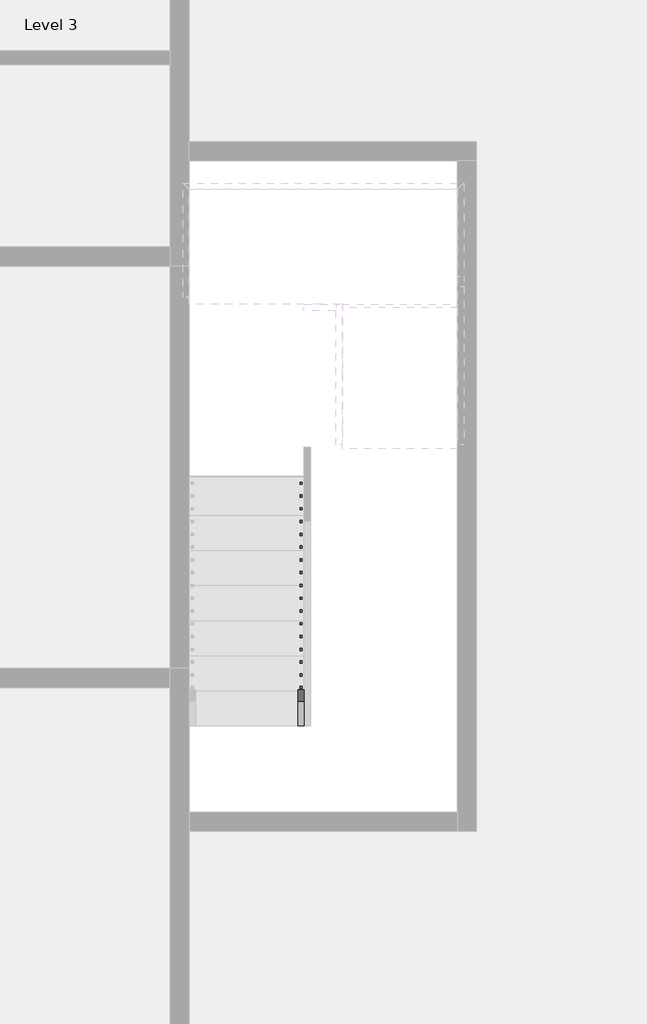
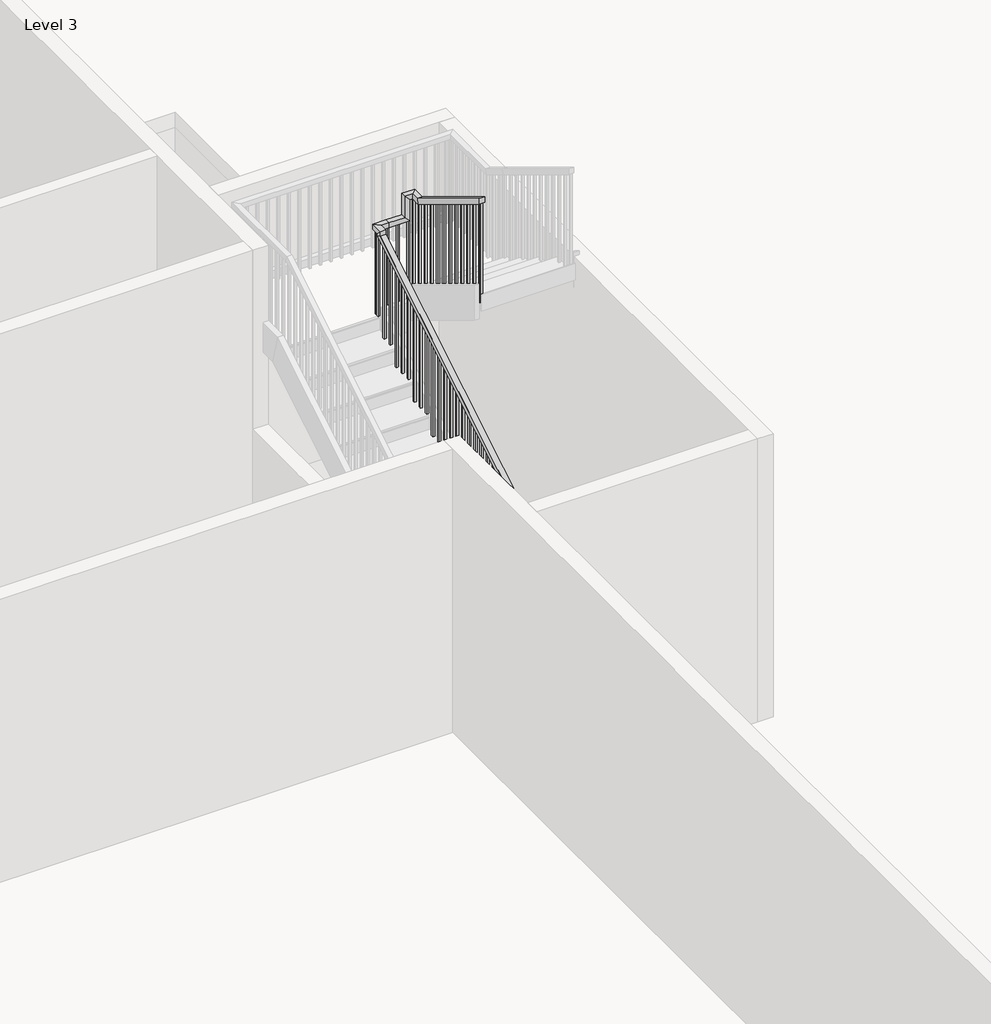
# One storey, part 7 of 8: 1 railing.
"""IFC4 building model written with IfcOpenShell, lengths in millimetres."""

from ifc_helpers import new_model, si_unit, frame, origin, place, context, project, spatial, polyline, outline, extrude, faceted_brep, element, save

model = new_model("IFC4")

# Units and contexts
model_context = context("Model", 3, world=origin())
ifc_project = project(units=[si_unit("LENGTHUNIT", "METRE", prefix="MILLI")], contexts=[model_context])

# Site, building, storey
site = spatial("IfcSite", under=ifc_project)
building = spatial("IfcBuilding", under=site)
storey = spatial("IfcBuildingStorey", under=building, Name="Level 3", Elevation=31330.6172466)

# Railing
placement = place(None, origin())
element("IfcRailing", 1, ObjectType="Handrail - Rectangular", at=placement, inside=storey, context=model_context, shape_type="SolidModel", body=[
    faceted_brep([(-2753.8415084, 19841.9216096, 32414.3505799), (-2753.8415084, 19841.9216096, 32354.9491197), (-2703.0415084, 19841.9216096, 32354.9491197), (-2703.0415084, 19841.9216096, 32414.3505799), (-2753.8415084, 23118.5216096, 34400.1687618), (-2753.8415084, 23169.3216096, 34371.5551803), (-2703.0415084, 23169.3216096, 34371.5551803), (-2703.0415084, 23118.5216096, 34400.1687618), (-2753.8415084, 23118.5216096, 34446.3505799), (-2753.8415084, 23169.3216096, 34395.5505799), (-2703.0415084, 23169.3216096, 34395.5505799), (-2703.0415084, 23118.5216096, 34446.3505799), (-2753.8415084, 23245.5216096, 34446.3505799), (-2753.8415084, 23245.5216096, 34395.5505799), (-2703.0415084, 23194.7216096, 34395.5505799), (-2703.0415084, 23194.7216096, 34446.3505799), (-2626.8415084, 23245.5216096, 34446.3505799), (-2626.8415084, 23245.5216096, 34395.5505799), (-2626.8415084, 23194.7216096, 34395.5505799), (-2626.8415084, 23194.7216096, 34446.3505799), (-2474.4415084, 23245.5216096, 34446.3505799), (-2423.6415084, 23245.5216096, 34395.5505799), (-2423.6415084, 23194.7216096, 34395.5505799), (-2474.4415084, 23194.7216096, 34446.3505799), (-2474.4415084, 23245.5216096, 34661.8657314), (-2423.6415084, 23245.5216096, 34611.0657314), (-2423.6415084, 23194.7216096, 34611.0657314), (-2474.4415084, 23194.7216096, 34661.8657314), (-2347.4415084, 23245.5216096, 34661.8657314), (-2347.4415084, 23245.5216096, 34611.0657314), (-2398.2415084, 23194.7216096, 34611.0657314), (-2398.2415084, 23194.7216096, 34661.8657314), (-2347.4415084, 23118.5216096, 34661.8657314), (-2347.4415084, 23104.3292002, 34611.0657314), (-2398.2415084, 23104.3292002, 34611.0657314), (-2398.2415084, 23118.5216096, 34661.8657314), (-2347.4415084, 22077.1216096, 35293.0172466), (-2398.2415084, 22077.1216096, 35293.0172466), (-2398.2415084, 22077.1216096, 35233.6157863), (-2347.4415084, 22077.1216096, 35233.6157863)], [[[0, 1, 2, 3]], [[1, 0, 4, 5]], [[2, 1, 5, 6]], [[3, 2, 6, 7]], [[0, 3, 7, 4]], [[5, 4, 8, 9]], [[6, 5, 9, 10]], [[7, 6, 10, 11]], [[4, 7, 11, 8]], [[9, 8, 12, 13]], [[10, 9, 13, 14]], [[11, 10, 14, 15]], [[8, 11, 15, 12]], [[13, 12, 16, 17]], [[14, 13, 17, 18]], [[15, 14, 18, 19]], [[12, 15, 19, 16]], [[17, 16, 20, 21]], [[18, 17, 21, 22]], [[19, 18, 22, 23]], [[16, 19, 23, 20]], [[21, 20, 24, 25]], [[22, 21, 25, 26]], [[23, 22, 26, 27]], [[20, 23, 27, 24]], [[25, 24, 28, 29]], [[26, 25, 29, 30]], [[27, 26, 30, 31]], [[24, 27, 31, 28]], [[29, 28, 32, 33]], [[30, 29, 33, 34]], [[31, 30, 34, 35]], [[28, 31, 35, 32]], [[36, 37, 38, 39]], [[33, 32, 36, 39]], [[34, 33, 39, 38]], [[35, 34, 38, 37]], [[32, 35, 37, 36]]]),
    extrude(outline(polyline([(22092.9966096, 35223.9945742), (22112.0466096, 35212.4491197), (22112.0466096, 34209.2839133), (22092.9966096, 34209.2839133), (22092.9966096, 35223.9945742)])), frame((-2382.3665084, 0.0, 0.0), z_axis=(1.0, 0.0, 0.0), x_axis=(0.0, 1.0, 0.0)), (0.0, 0.0, 1.0), 19.05),
    extrude(outline(polyline([(22194.5966096, 35162.4188166), (22213.6466096, 35150.8733621), (22213.6466096, 34209.2839133), (22194.5966096, 34209.2839133), (22194.5966096, 35162.4188166)])), frame((-2382.3665084, 0.0, 0.0), z_axis=(1.0, 0.0, 0.0), x_axis=(0.0, 1.0, 0.0)), (0.0, 0.0, 1.0), 19.05),
    extrude(outline(polyline([(22296.1966096, 35100.8430591), (22315.2466096, 35089.2976045), (22315.2466096, 34209.2839133), (22296.1966096, 34209.2839133), (22296.1966096, 35100.8430591)])), frame((-2382.3665084, 0.0, 0.0), z_axis=(1.0, 0.0, 0.0), x_axis=(0.0, 1.0, 0.0)), (0.0, 0.0, 1.0), 19.05),
    extrude(outline(polyline([(22397.7966096, 35039.2673015), (22416.8466096, 35027.721847), (22416.8466096, 34039.9505799), (22397.7966096, 34039.9505799), (22397.7966096, 35039.2673015)])), frame((-2382.3665084, 0.0, 0.0), z_axis=(1.0, 0.0, 0.0), x_axis=(0.0, 1.0, 0.0)), (0.0, 0.0, 1.0), 19.05),
    extrude(outline(polyline([(22499.3966096, 34977.6915439), (22518.4466096, 34966.1460894), (22518.4466096, 34039.9505799), (22499.3966096, 34039.9505799), (22499.3966096, 34977.6915439)])), frame((-2382.3665084, 0.0, 0.0), z_axis=(1.0, 0.0, 0.0), x_axis=(0.0, 1.0, 0.0)), (0.0, 0.0, 1.0), 19.05),
    extrude(outline(polyline([(22600.9966096, 34916.1157863), (22620.0466096, 34904.5703318), (22620.0466096, 34039.9505799), (22600.9966096, 34039.9505799), (22600.9966096, 34916.1157863)])), frame((-2382.3665084, 0.0, 0.0), z_axis=(1.0, 0.0, 0.0), x_axis=(0.0, 1.0, 0.0)), (0.0, 0.0, 1.0), 19.05),
    extrude(outline(polyline([(22702.5966096, 34854.5400288), (22721.6466096, 34842.9945742), (22721.6466096, 33870.6172466), (22702.5966096, 33870.6172466), (22702.5966096, 34854.5400288)])), frame((-2382.3665084, 0.0, 0.0), z_axis=(1.0, 0.0, 0.0), x_axis=(0.0, 1.0, 0.0)), (0.0, 0.0, 1.0), 19.05),
    extrude(outline(polyline([(22804.1966096, 34792.9642712), (22823.2466096, 34781.4188166), (22823.2466096, 33870.6172466), (22804.1966096, 33870.6172466), (22804.1966096, 34792.9642712)])), frame((-2382.3665084, 0.0, 0.0), z_axis=(1.0, 0.0, 0.0), x_axis=(0.0, 1.0, 0.0)), (0.0, 0.0, 1.0), 19.05),
    extrude(outline(polyline([(22905.7966096, 34731.3885136), (22924.8466096, 34719.8430591), (22924.8466096, 33870.6172466), (22905.7966096, 33870.6172466), (22905.7966096, 34731.3885136)])), frame((-2382.3665084, 0.0, 0.0), z_axis=(1.0, 0.0, 0.0), x_axis=(0.0, 1.0, 0.0)), (0.0, 0.0, 1.0), 19.05),
    extrude(outline(polyline([(23007.3966096, 34669.812756), (23026.4466096, 34658.2673015), (23026.4466096, 33701.2839133), (23007.3966096, 33701.2839133), (23007.3966096, 34669.812756)])), frame((-2382.3665084, 0.0, 0.0), z_axis=(1.0, 0.0, 0.0), x_axis=(0.0, 1.0, 0.0)), (0.0, 0.0, 1.0), 19.05),
    extrude(outline(polyline([(23108.9966096, 34608.2369985), (23128.0466096, 34596.6915439), (23128.0466096, 33701.2839133), (23108.9966096, 33701.2839133), (23108.9966096, 34608.2369985)])), frame((-2382.3665084, 0.0, 0.0), z_axis=(1.0, 0.0, 0.0), x_axis=(0.0, 1.0, 0.0)), (0.0, 0.0, 1.0), 19.05),
    extrude(outline(polyline([(-2433.1665084, 23210.5966096), (-2433.1665084, 23229.6466096), (-2414.1165084, 23229.6466096), (-2414.1165084, 23210.5966096), (-2433.1665084, 23210.5966096)])), frame((0.0, 0.0, 33531.9505799), z_axis=(0.0, 0.0, 1.0), x_axis=(1.0, 0.0, 0.0)), (0.0, 0.0, 1.0), 1079.1151515),
    extrude(outline(polyline([(-2534.7665084, 23210.5966096), (-2534.7665084, 23229.6466096), (-2515.7165084, 23229.6466096), (-2515.7165084, 23210.5966096), (-2534.7665084, 23210.5966096)])), frame((0.0, 0.0, 33531.9505799), z_axis=(0.0, 0.0, 1.0), x_axis=(1.0, 0.0, 0.0)), (0.0, 0.0, 1.0), 863.6),
    extrude(outline(polyline([(-2636.3665084, 23210.5966096), (-2636.3665084, 23229.6466096), (-2617.3165084, 23229.6466096), (-2617.3165084, 23210.5966096), (-2636.3665084, 23210.5966096)])), frame((0.0, 0.0, 33531.9505799), z_axis=(0.0, 0.0, 1.0), x_axis=(1.0, 0.0, 0.0)), (0.0, 0.0, 1.0), 863.6),
    extrude(outline(polyline([(-2718.9165084, 23185.1966096), (-2737.9665084, 23185.1966096), (-2737.9665084, 23204.2466096), (-2718.9165084, 23204.2466096), (-2718.9165084, 23185.1966096)])), frame((0.0, 0.0, 33531.9505799), z_axis=(0.0, 0.0, 1.0), x_axis=(1.0, 0.0, 0.0)), (0.0, 0.0, 1.0), 863.6),
    extrude(outline(polyline([(23083.5966096, 34319.6006348), (23102.6466096, 34331.1460894), (23102.6466096, 33362.6172466), (23083.5966096, 33362.6172466), (23083.5966096, 34319.6006348)])), frame((-2737.9665084, 0.0, 0.0), z_axis=(1.0, 0.0, 0.0), x_axis=(0.0, 1.0, 0.0)), (0.0, 0.0, 1.0), 19.05),
    extrude(outline(polyline([(22981.9966096, 34258.0248773), (23001.0466096, 34269.5703318), (23001.0466096, 33362.6172466), (22981.9966096, 33362.6172466), (22981.9966096, 34258.0248773)])), frame((-2737.9665084, 0.0, 0.0), z_axis=(1.0, 0.0, 0.0), x_axis=(0.0, 1.0, 0.0)), (0.0, 0.0, 1.0), 19.05),
    extrude(outline(polyline([(22880.3966096, 34196.4491197), (22899.4466096, 34207.9945742), (22899.4466096, 33193.2839133), (22880.3966096, 33193.2839133), (22880.3966096, 34196.4491197)])), frame((-2737.9665084, 0.0, 0.0), z_axis=(1.0, 0.0, 0.0), x_axis=(0.0, 1.0, 0.0)), (0.0, 0.0, 1.0), 19.05),
    extrude(outline(polyline([(22778.7966096, 34134.8733621), (22797.8466096, 34146.4188166), (22797.8466096, 33193.2839133), (22778.7966096, 33193.2839133), (22778.7966096, 34134.8733621)])), frame((-2737.9665084, 0.0, 0.0), z_axis=(1.0, 0.0, 0.0), x_axis=(0.0, 1.0, 0.0)), (0.0, 0.0, 1.0), 19.05),
    extrude(outline(polyline([(22677.1966096, 34073.2976045), (22696.2466096, 34084.8430591), (22696.2466096, 33193.2839133), (22677.1966096, 33193.2839133), (22677.1966096, 34073.2976045)])), frame((-2737.9665084, 0.0, 0.0), z_axis=(1.0, 0.0, 0.0), x_axis=(0.0, 1.0, 0.0)), (0.0, 0.0, 1.0), 19.05),
    extrude(outline(polyline([(22575.5966096, 34011.721847), (22594.6466096, 34023.2673015), (22594.6466096, 33023.9505799), (22575.5966096, 33023.9505799), (22575.5966096, 34011.721847)])), frame((-2737.9665084, 0.0, 0.0), z_axis=(1.0, 0.0, 0.0), x_axis=(0.0, 1.0, 0.0)), (0.0, 0.0, 1.0), 19.05),
    extrude(outline(polyline([(22473.9966096, 33950.1460894), (22493.0466096, 33961.6915439), (22493.0466096, 33023.9505799), (22473.9966096, 33023.9505799), (22473.9966096, 33950.1460894)])), frame((-2737.9665084, 0.0, 0.0), z_axis=(1.0, 0.0, 0.0), x_axis=(0.0, 1.0, 0.0)), (0.0, 0.0, 1.0), 19.05),
    extrude(outline(polyline([(22372.3966096, 33888.5703318), (22391.4466096, 33900.1157863), (22391.4466096, 33023.9505799), (22372.3966096, 33023.9505799), (22372.3966096, 33888.5703318)])), frame((-2737.9665084, 0.0, 0.0), z_axis=(1.0, 0.0, 0.0), x_axis=(0.0, 1.0, 0.0)), (0.0, 0.0, 1.0), 19.05),
    extrude(outline(polyline([(22270.7966096, 33826.9945742), (22289.8466096, 33838.5400288), (22289.8466096, 32854.6172466), (22270.7966096, 32854.6172466), (22270.7966096, 33826.9945742)])), frame((-2737.9665084, 0.0, 0.0), z_axis=(1.0, 0.0, 0.0), x_axis=(0.0, 1.0, 0.0)), (0.0, 0.0, 1.0), 19.05),
    extrude(outline(polyline([(22169.1966096, 33765.4188166), (22188.2466096, 33776.9642712), (22188.2466096, 32854.6172466), (22169.1966096, 32854.6172466), (22169.1966096, 33765.4188166)])), frame((-2737.9665084, 0.0, 0.0), z_axis=(1.0, 0.0, 0.0), x_axis=(0.0, 1.0, 0.0)), (0.0, 0.0, 1.0), 19.05),
    extrude(outline(polyline([(22067.5966096, 33703.8430591), (22086.6466096, 33715.3885136), (22086.6466096, 32854.6172466), (22067.5966096, 32854.6172466), (22067.5966096, 33703.8430591)])), frame((-2737.9665084, 0.0, 0.0), z_axis=(1.0, 0.0, 0.0), x_axis=(0.0, 1.0, 0.0)), (0.0, 0.0, 1.0), 19.05),
    extrude(outline(polyline([(21965.9966096, 33642.2673015), (21985.0466096, 33653.812756), (21985.0466096, 32685.2839133), (21965.9966096, 32685.2839133), (21965.9966096, 33642.2673015)])), frame((-2737.9665084, 0.0, 0.0), z_axis=(1.0, 0.0, 0.0), x_axis=(0.0, 1.0, 0.0)), (0.0, 0.0, 1.0), 19.05),
    extrude(outline(polyline([(21864.3966096, 33580.6915439), (21883.4466096, 33592.2369985), (21883.4466096, 32685.2839133), (21864.3966096, 32685.2839133), (21864.3966096, 33580.6915439)])), frame((-2737.9665084, 0.0, 0.0), z_axis=(1.0, 0.0, 0.0), x_axis=(0.0, 1.0, 0.0)), (0.0, 0.0, 1.0), 19.05),
    extrude(outline(polyline([(21762.7966096, 33519.1157863), (21781.8466096, 33530.6612409), (21781.8466096, 32515.9505799), (21762.7966096, 32515.9505799), (21762.7966096, 33519.1157863)])), frame((-2737.9665084, 0.0, 0.0), z_axis=(1.0, 0.0, 0.0), x_axis=(0.0, 1.0, 0.0)), (0.0, 0.0, 1.0), 19.05),
    extrude(outline(polyline([(21661.1966096, 33457.5400288), (21680.2466096, 33469.0854833), (21680.2466096, 32515.9505799), (21661.1966096, 32515.9505799), (21661.1966096, 33457.5400288)])), frame((-2737.9665084, 0.0, 0.0), z_axis=(1.0, 0.0, 0.0), x_axis=(0.0, 1.0, 0.0)), (0.0, 0.0, 1.0), 19.05),
    extrude(outline(polyline([(21559.5966096, 33395.9642712), (21578.6466096, 33407.5097257), (21578.6466096, 32515.9505799), (21559.5966096, 32515.9505799), (21559.5966096, 33395.9642712)])), frame((-2737.9665084, 0.0, 0.0), z_axis=(1.0, 0.0, 0.0), x_axis=(0.0, 1.0, 0.0)), (0.0, 0.0, 1.0), 19.05),
    extrude(outline(polyline([(21457.9966096, 33334.3885136), (21477.0466096, 33345.9339682), (21477.0466096, 32346.6172466), (21457.9966096, 32346.6172466), (21457.9966096, 33334.3885136)])), frame((-2737.9665084, 0.0, 0.0), z_axis=(1.0, 0.0, 0.0), x_axis=(0.0, 1.0, 0.0)), (0.0, 0.0, 1.0), 19.05),
    extrude(outline(polyline([(21356.3966096, 33272.812756), (21375.4466096, 33284.3582106), (21375.4466096, 32346.6172466), (21356.3966096, 32346.6172466), (21356.3966096, 33272.812756)])), frame((-2737.9665084, 0.0, 0.0), z_axis=(1.0, 0.0, 0.0), x_axis=(0.0, 1.0, 0.0)), (0.0, 0.0, 1.0), 19.05),
    extrude(outline(polyline([(21254.7966096, 33211.2369985), (21273.8466096, 33222.782453), (21273.8466096, 32346.6172466), (21254.7966096, 32346.6172466), (21254.7966096, 33211.2369985)])), frame((-2737.9665084, 0.0, 0.0), z_axis=(1.0, 0.0, 0.0), x_axis=(0.0, 1.0, 0.0)), (0.0, 0.0, 1.0), 19.05),
    extrude(outline(polyline([(21153.1966096, 33149.6612409), (21172.2466096, 33161.2066954), (21172.2466096, 32177.2839133), (21153.1966096, 32177.2839133), (21153.1966096, 33149.6612409)])), frame((-2737.9665084, 0.0, 0.0), z_axis=(1.0, 0.0, 0.0), x_axis=(0.0, 1.0, 0.0)), (0.0, 0.0, 1.0), 19.05),
    extrude(outline(polyline([(21051.5966096, 33088.0854833), (21070.6466096, 33099.6309379), (21070.6466096, 32177.2839133), (21051.5966096, 32177.2839133), (21051.5966096, 33088.0854833)])), frame((-2737.9665084, 0.0, 0.0), z_axis=(1.0, 0.0, 0.0), x_axis=(0.0, 1.0, 0.0)), (0.0, 0.0, 1.0), 19.05),
    extrude(outline(polyline([(20949.9966096, 33026.5097257), (20969.0466096, 33038.0551803), (20969.0466096, 32177.2839133), (20949.9966096, 32177.2839133), (20949.9966096, 33026.5097257)])), frame((-2737.9665084, 0.0, 0.0), z_axis=(1.0, 0.0, 0.0), x_axis=(0.0, 1.0, 0.0)), (0.0, 0.0, 1.0), 19.05),
    extrude(outline(polyline([(20848.3966096, 32964.9339682), (20867.4466096, 32976.4794227), (20867.4466096, 32007.9505799), (20848.3966096, 32007.9505799), (20848.3966096, 32964.9339682)])), frame((-2737.9665084, 0.0, 0.0), z_axis=(1.0, 0.0, 0.0), x_axis=(0.0, 1.0, 0.0)), (0.0, 0.0, 1.0), 19.05),
    extrude(outline(polyline([(20746.7966096, 32903.3582106), (20765.8466096, 32914.9036651), (20765.8466096, 32007.9505799), (20746.7966096, 32007.9505799), (20746.7966096, 32903.3582106)])), frame((-2737.9665084, 0.0, 0.0), z_axis=(1.0, 0.0, 0.0), x_axis=(0.0, 1.0, 0.0)), (0.0, 0.0, 1.0), 19.05),
    extrude(outline(polyline([(20645.1966096, 32841.782453), (20664.2466096, 32853.3279076), (20664.2466096, 31838.6172466), (20645.1966096, 31838.6172466), (20645.1966096, 32841.782453)])), frame((-2737.9665084, 0.0, 0.0), z_axis=(1.0, 0.0, 0.0), x_axis=(0.0, 1.0, 0.0)), (0.0, 0.0, 1.0), 19.05),
    extrude(outline(polyline([(20543.5966096, 32780.2066954), (20562.6466096, 32791.75215), (20562.6466096, 31838.6172466), (20543.5966096, 31838.6172466), (20543.5966096, 32780.2066954)])), frame((-2737.9665084, 0.0, 0.0), z_axis=(1.0, 0.0, 0.0), x_axis=(0.0, 1.0, 0.0)), (0.0, 0.0, 1.0), 19.05),
    extrude(outline(polyline([(20441.9966096, 32718.6309379), (20461.0466096, 32730.1763924), (20461.0466096, 31838.6172466), (20441.9966096, 31838.6172466), (20441.9966096, 32718.6309379)])), frame((-2737.9665084, 0.0, 0.0), z_axis=(1.0, 0.0, 0.0), x_axis=(0.0, 1.0, 0.0)), (0.0, 0.0, 1.0), 19.05),
    extrude(outline(polyline([(20340.3966096, 32657.0551803), (20359.4466096, 32668.6006348), (20359.4466096, 31669.2839133), (20340.3966096, 31669.2839133), (20340.3966096, 32657.0551803)])), frame((-2737.9665084, 0.0, 0.0), z_axis=(1.0, 0.0, 0.0), x_axis=(0.0, 1.0, 0.0)), (0.0, 0.0, 1.0), 19.05),
    extrude(outline(polyline([(20238.7966096, 32595.4794227), (20257.8466096, 32607.0248773), (20257.8466096, 31669.2839133), (20238.7966096, 31669.2839133), (20238.7966096, 32595.4794227)])), frame((-2737.9665084, 0.0, 0.0), z_axis=(1.0, 0.0, 0.0), x_axis=(0.0, 1.0, 0.0)), (0.0, 0.0, 1.0), 19.05),
    extrude(outline(polyline([(20137.1966096, 32533.9036651), (20156.2466096, 32545.4491197), (20156.2466096, 31669.2839133), (20137.1966096, 31669.2839133), (20137.1966096, 32533.9036651)])), frame((-2737.9665084, 0.0, 0.0), z_axis=(1.0, 0.0, 0.0), x_axis=(0.0, 1.0, 0.0)), (0.0, 0.0, 1.0), 19.05),
    extrude(outline(polyline([(20035.5966096, 32472.3279076), (20054.6466096, 32483.8733621), (20054.6466096, 31499.9505799), (20035.5966096, 31499.9505799), (20035.5966096, 32472.3279076)])), frame((-2737.9665084, 0.0, 0.0), z_axis=(1.0, 0.0, 0.0), x_axis=(0.0, 1.0, 0.0)), (0.0, 0.0, 1.0), 19.05),
    extrude(outline(polyline([(19933.9966096, 32410.75215), (19953.0466096, 32422.2976045), (19953.0466096, 31499.9505799), (19933.9966096, 31499.9505799), (19933.9966096, 32410.75215)])), frame((-2737.9665084, 0.0, 0.0), z_axis=(1.0, 0.0, 0.0), x_axis=(0.0, 1.0, 0.0)), (0.0, 0.0, 1.0), 19.05),
    extrude(outline(polyline([(-2382.3665084, 23210.5966096), (-2382.3665084, 23229.6466096), (-2363.3165084, 23229.6466096), (-2363.3165084, 23210.5966096), (-2382.3665084, 23210.5966096)])), frame((0.0, 0.0, 33531.9505799), z_axis=(0.0, 0.0, 1.0), x_axis=(1.0, 0.0, 0.0)), (0.0, 0.0, 1.0), 1079.1151515),
    extrude(outline(polyline([(-2718.9165084, 23210.5966096), (-2737.9665084, 23210.5966096), (-2737.9665084, 23229.6466096), (-2718.9165084, 23229.6466096), (-2718.9165084, 23210.5966096)])), frame((0.0, 0.0, 33531.9505799), z_axis=(0.0, 0.0, 1.0), x_axis=(1.0, 0.0, 0.0)), (0.0, 0.0, 1.0), 863.6),
    extrude(outline(polyline([(22077.1216096, 35233.6157863), (22096.1716096, 35222.0703318), (22096.1716096, 34209.2839133), (22077.1216096, 34209.2839133), (22077.1216096, 35233.6157863)])), frame((-2382.3665084, 0.0, 0.0), z_axis=(1.0, 0.0, 0.0), x_axis=(0.0, 1.0, 0.0)), (0.0, 0.0, 1.0), 19.05),
    extrude(outline(polyline([(19841.9216096, 32354.9491197), (19860.9716096, 32366.4945742), (19860.9716096, 31499.9505799), (19841.9216096, 31499.9505799), (19841.9216096, 32354.9491197)])), frame((-2737.9665084, 0.0, 0.0), z_axis=(1.0, 0.0, 0.0), x_axis=(0.0, 1.0, 0.0)), (0.0, 0.0, 1.0), 19.05),
])

save(model, "model.ifc")

# Revit data of these elements
# Type "Handrail - Rectangular"
#   Assembly Code = "C2010400"
#   built-in parameter 1008612 = 0.0416667 (stored number, unit not read)
#   built-in parameter 1008611 = 0.0416667 (stored number, unit not read)
#   built-in parameter 1008609 = 0.333333 (stored number, unit not read)
#   built-in parameter 1008604 = 0.166667 (stored number, unit not read)
#   built-in parameter 1008603 = 0.166667 (stored number, unit not read)
#   Railing Height = 3' - 0"
#   built-in parameter 1008630 = 2
#   built-in parameter 1008610 = 2
#   built-in parameter 1008618 = Baluster - Square : 3/4"
# Element 1 (IfcRailing, "Handrail - Rectangular")
#   Phase Created = New Construction
